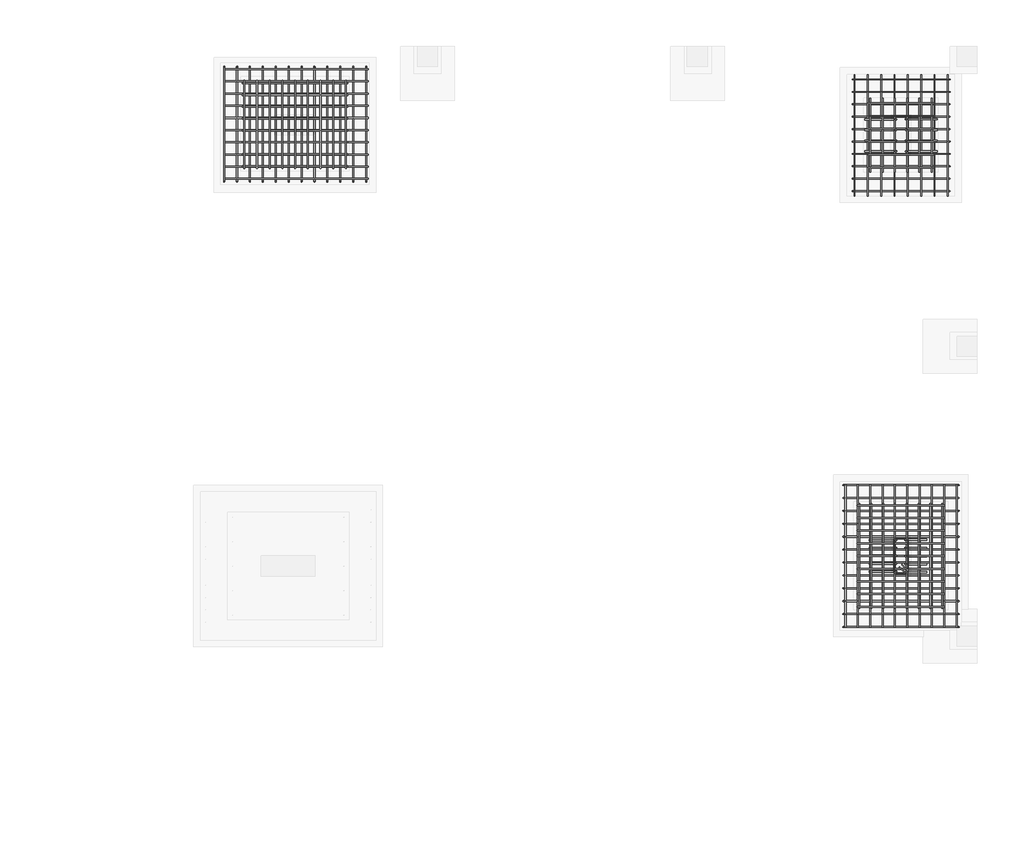
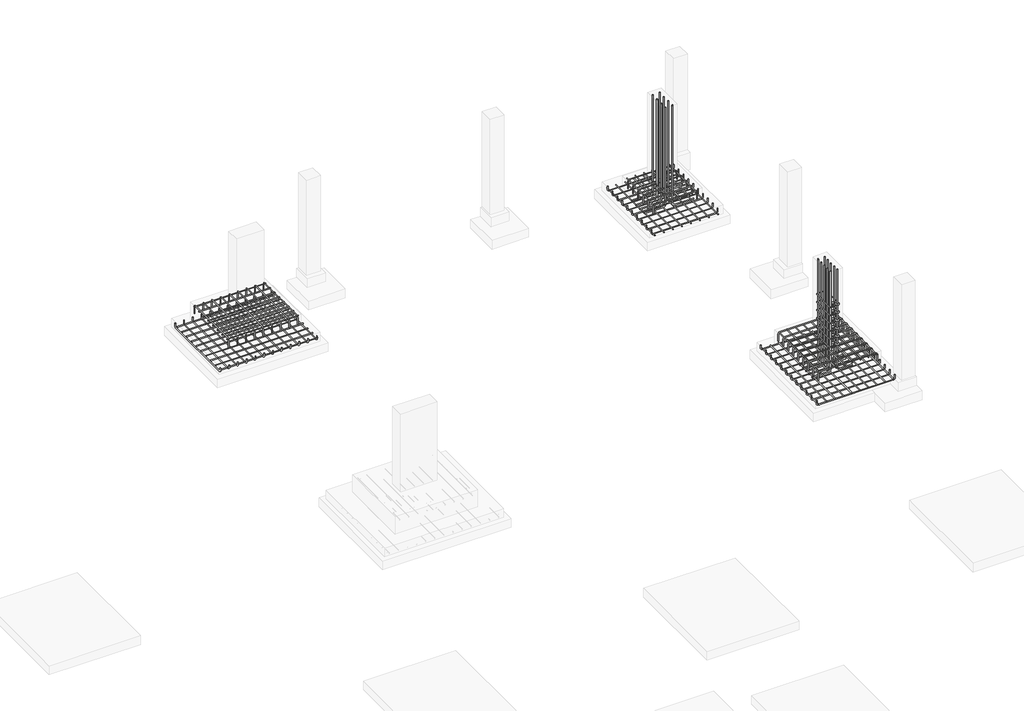
# One storey, part 6 of 6: 17 reinforcing bars.
"""IFC4 building model written with IfcOpenShell, lengths in millimetres."""

from ifc_helpers import new_model, si_unit, point, frame, origin, place, context, project, spatial, polyline, circle_curve, trimmed, segment, composite_curve, source, transform, mapped, element, save
from ifc_brep_helpers import swept_disk

model = new_model("IFC4")

# Units and contexts
model_context = context("Model", 3, world=origin())
ifc_project = project(units=[si_unit("LENGTHUNIT", "METRE", prefix="MILLI")], contexts=[model_context])

# Site, building, storey
site = spatial("IfcSite", under=ifc_project)
building = spatial("IfcBuilding", under=site)
storey = spatial("IfcBuildingStorey", under=building, Elevation=-1828.8)

# Reinforcing bars
placement = place(None, origin())
reinforcing_bar_shape = source(origin(), model_context, "Body", "SolidModel", [
    swept_disk(composite_curve([segment(polyline([(5668412.2527589, -3584746.7384702, -1801.3373708), (5670028.6527589, -3584746.7384702, -1801.3373708)]), True, "CONTINUOUS")], self_intersect=False), 6.0),
])
element("IfcReinforcingBar", 1, at=placement, inside=storey, context=model_context, shape_type="MappedRepresentation", body=[
    mapped(reinforcing_bar_shape, transform((0.0, 0.0, 0.0), x_axis=(1.0, 0.0, 0.0), y_axis=(0.0, 1.0, 0.0), z_axis=(0.0, 0.0, 1.0))),
    mapped(reinforcing_bar_shape, transform((0.0, -137.644158, 0.0), x_axis=(1.0, 0.0, 0.0), y_axis=(0.0, 1.0, 0.0), z_axis=(0.0, 0.0, 1.0))),
    mapped(reinforcing_bar_shape, transform((0.0, -275.2883159, 0.0), x_axis=(1.0, 0.0, 0.0), y_axis=(0.0, 1.0, 0.0), z_axis=(0.0, 0.0, 1.0))),
    mapped(reinforcing_bar_shape, transform((0.0, -412.9324739, 0.0), x_axis=(1.0, 0.0, 0.0), y_axis=(0.0, 1.0, 0.0), z_axis=(0.0, 0.0, 1.0))),
    mapped(reinforcing_bar_shape, transform((0.0, -550.5766318, 0.0), x_axis=(1.0, 0.0, 0.0), y_axis=(0.0, 1.0, 0.0), z_axis=(0.0, 0.0, 1.0))),
    mapped(reinforcing_bar_shape, transform((0.0, -688.2207898, 0.0), x_axis=(1.0, 0.0, 0.0), y_axis=(0.0, 1.0, 0.0), z_axis=(0.0, 0.0, 1.0))),
    mapped(reinforcing_bar_shape, transform((0.0, -825.8649477, 0.0), x_axis=(1.0, 0.0, 0.0), y_axis=(0.0, 1.0, 0.0), z_axis=(0.0, 0.0, 1.0))),
    mapped(reinforcing_bar_shape, transform((0.0, -963.5091057, 0.0), x_axis=(1.0, 0.0, 0.0), y_axis=(0.0, 1.0, 0.0), z_axis=(0.0, 0.0, 1.0))),
    mapped(reinforcing_bar_shape, transform((0.0, -1101.1532636, 0.0), x_axis=(1.0, 0.0, 0.0), y_axis=(0.0, 1.0, 0.0), z_axis=(0.0, 0.0, 1.0))),
    mapped(reinforcing_bar_shape, transform((0.0, -1238.7974216, 0.0), x_axis=(1.0, 0.0, 0.0), y_axis=(0.0, 1.0, 0.0), z_axis=(0.0, 0.0, 1.0))),
])
reinforcing_bar_2_shape = source(origin(), model_context, "Body", "SolidModel", [
    swept_disk(composite_curve([segment(polyline([(5669774.8297535, -3585864.1224803, -1551.6), (5669774.8297535, -3585864.1224803, -1437.6)]), True, "CONTINUOUS"), segment(trimmed(circle_curve(frame((5669774.8297535, -3585834.1224803, -1437.6), z_axis=(-1.0, 0.0, 0.0), x_axis=(0.0, -30.0, 0.0)), 30.0), [point((5669774.8297535, -3585864.1224803, -1437.6))], [point((5669774.8297535, -3585834.1224803, -1407.6))], True, "CARTESIAN"), True, "CONTINUOUS"), segment(polyline([(5669774.8297535, -3585834.1224803, -1407.6), (5669774.8297535, -3584907.6254563, -1407.6)]), True, "CONTINUOUS"), segment(trimmed(circle_curve(frame((5669774.8297535, -3584907.6254563, -1437.6), z_axis=(-1.0, 0.0, 0.0), x_axis=(0.0, 0.0, 30.0)), 30.0), [point((5669774.8297535, -3584907.6254563, -1407.6))], [point((5669774.8297535, -3584877.6254563, -1437.6))], True, "CARTESIAN"), True, "CONTINUOUS"), segment(polyline([(5669774.8297535, -3584877.6254563, -1437.6), (5669774.8297535, -3584877.6254563, -1551.6)]), True, "CONTINUOUS")], self_intersect=False), 6.0),
])
element("IfcReinforcingBar", 2, at=placement, inside=storey, context=model_context, shape_type="MappedRepresentation", body=[
    mapped(reinforcing_bar_2_shape, transform((0.0, 0.0, 0.0), x_axis=(1.0, 0.0, 0.0), y_axis=(0.0, 1.0, 0.0), z_axis=(0.0, 0.0, 1.0))),
    mapped(reinforcing_bar_2_shape, transform((-143.4, 0.0, 0.0), x_axis=(1.0, 0.0, 0.0), y_axis=(0.0, 1.0, 0.0), z_axis=(0.0, 0.0, 1.0))),
    mapped(reinforcing_bar_2_shape, transform((-286.8, 0.0, 0.0), x_axis=(1.0, 0.0, 0.0), y_axis=(0.0, 1.0, 0.0), z_axis=(0.0, 0.0, 1.0))),
    mapped(reinforcing_bar_2_shape, transform((-430.2, 0.0, 0.0), x_axis=(1.0, 0.0, 0.0), y_axis=(0.0, 1.0, 0.0), z_axis=(0.0, 0.0, 1.0))),
    mapped(reinforcing_bar_2_shape, transform((-573.6, 0.0, 0.0), x_axis=(1.0, 0.0, 0.0), y_axis=(0.0, 1.0, 0.0), z_axis=(0.0, 0.0, 1.0))),
    mapped(reinforcing_bar_2_shape, transform((-717.0, 0.0, 0.0), x_axis=(1.0, 0.0, 0.0), y_axis=(0.0, 1.0, 0.0), z_axis=(0.0, 0.0, 1.0))),
    mapped(reinforcing_bar_2_shape, transform((-860.4, 0.0, 0.0), x_axis=(1.0, 0.0, 0.0), y_axis=(0.0, 1.0, 0.0), z_axis=(0.0, 0.0, 1.0))),
    mapped(reinforcing_bar_2_shape, transform((-1003.8, 0.0, 0.0), x_axis=(1.0, 0.0, 0.0), y_axis=(0.0, 1.0, 0.0), z_axis=(0.0, 0.0, 1.0))),
    mapped(reinforcing_bar_2_shape, transform((-1147.2, 0.0, 0.0), x_axis=(1.0, 0.0, 0.0), y_axis=(0.0, 1.0, 0.0), z_axis=(0.0, 0.0, 1.0))),
])
reinforcing_bar_3_shape = source(origin(), model_context, "Body", "SolidModel", [
    swept_disk(composite_curve([segment(polyline([(5669794.2997613, -3585840.5657222, -1419.7151301), (5668606.7353359, -3585840.5657222, -1419.7151301)]), True, "CONTINUOUS")], self_intersect=False), 6.0),
])
element("IfcReinforcingBar", 3, at=placement, inside=storey, context=model_context, shape_type="MappedRepresentation", body=[
    mapped(reinforcing_bar_3_shape, transform((0.0, 0.0, 0.0), x_axis=(1.0, 0.0, 0.0), y_axis=(0.0, 1.0, 0.0), z_axis=(0.0, 0.0, 1.0))),
    mapped(reinforcing_bar_3_shape, transform((0.0, 133.8141, 0.0), x_axis=(1.0, 0.0, 0.0), y_axis=(0.0, 1.0, 0.0), z_axis=(0.0, 0.0, 1.0))),
    mapped(reinforcing_bar_3_shape, transform((0.0, 267.6282001, 0.0), x_axis=(1.0, 0.0, 0.0), y_axis=(0.0, 1.0, 0.0), z_axis=(0.0, 0.0, 1.0))),
    mapped(reinforcing_bar_3_shape, transform((0.0, 401.4423001, 0.0), x_axis=(1.0, 0.0, 0.0), y_axis=(0.0, 1.0, 0.0), z_axis=(0.0, 0.0, 1.0))),
    mapped(reinforcing_bar_3_shape, transform((0.0, 535.2564002, 0.0), x_axis=(1.0, 0.0, 0.0), y_axis=(0.0, 1.0, 0.0), z_axis=(0.0, 0.0, 1.0))),
    mapped(reinforcing_bar_3_shape, transform((0.0, 669.0705002, 0.0), x_axis=(1.0, 0.0, 0.0), y_axis=(0.0, 1.0, 0.0), z_axis=(0.0, 0.0, 1.0))),
    mapped(reinforcing_bar_3_shape, transform((0.0, 802.8846003, 0.0), x_axis=(1.0, 0.0, 0.0), y_axis=(0.0, 1.0, 0.0), z_axis=(0.0, 0.0, 1.0))),
    mapped(reinforcing_bar_3_shape, transform((0.0, 936.6987003, 0.0), x_axis=(1.0, 0.0, 0.0), y_axis=(0.0, 1.0, 0.0), z_axis=(0.0, 0.0, 1.0))),
])
reinforcing_bar_4_shape = source(origin(), model_context, "Body", "SolidModel", [
    swept_disk(composite_curve([segment(polyline([(5676673.9153747, -3589441.4682909, -1779.1123708), (5676673.9153747, -3591057.8682909, -1779.1123708)]), True, "CONTINUOUS")], self_intersect=False), 6.0),
])
element("IfcReinforcingBar", 4, at=placement, inside=storey, context=model_context, shape_type="MappedRepresentation", body=[
    mapped(reinforcing_bar_4_shape, transform((0.0, 0.0, 0.0), x_axis=(1.0, 0.0, 0.0), y_axis=(0.0, 1.0, 0.0), z_axis=(0.0, 0.0, 1.0))),
    mapped(reinforcing_bar_4_shape, transform((-139.3613026, 0.0, 0.0), x_axis=(1.0, 0.0, 0.0), y_axis=(0.0, 1.0, 0.0), z_axis=(0.0, 0.0, 1.0))),
    mapped(reinforcing_bar_4_shape, transform((-278.7226053, 0.0, 0.0), x_axis=(1.0, 0.0, 0.0), y_axis=(0.0, 1.0, 0.0), z_axis=(0.0, 0.0, 1.0))),
    mapped(reinforcing_bar_4_shape, transform((-418.0839079, 0.0, 0.0), x_axis=(1.0, 0.0, 0.0), y_axis=(0.0, 1.0, 0.0), z_axis=(0.0, 0.0, 1.0))),
    mapped(reinforcing_bar_4_shape, transform((-557.4452106, 0.0, 0.0), x_axis=(1.0, 0.0, 0.0), y_axis=(0.0, 1.0, 0.0), z_axis=(0.0, 0.0, 1.0))),
    mapped(reinforcing_bar_4_shape, transform((-696.8065132, 0.0, 0.0), x_axis=(1.0, 0.0, 0.0), y_axis=(0.0, 1.0, 0.0), z_axis=(0.0, 0.0, 1.0))),
    mapped(reinforcing_bar_4_shape, transform((-836.1678159, 0.0, 0.0), x_axis=(1.0, 0.0, 0.0), y_axis=(0.0, 1.0, 0.0), z_axis=(0.0, 0.0, 1.0))),
    mapped(reinforcing_bar_4_shape, transform((-975.5291185, 0.0, 0.0), x_axis=(1.0, 0.0, 0.0), y_axis=(0.0, 1.0, 0.0), z_axis=(0.0, 0.0, 1.0))),
    mapped(reinforcing_bar_4_shape, transform((-1114.8904212, 0.0, 0.0), x_axis=(1.0, 0.0, 0.0), y_axis=(0.0, 1.0, 0.0), z_axis=(0.0, 0.0, 1.0))),
    mapped(reinforcing_bar_4_shape, transform((-1254.2517238, 0.0, 0.0), x_axis=(1.0, 0.0, 0.0), y_axis=(0.0, 1.0, 0.0), z_axis=(0.0, 0.0, 1.0))),
])
reinforcing_bar_5_shape = source(origin(), model_context, "Body", "SolidModel", [
    swept_disk(composite_curve([segment(polyline([(5675555.1175203, -3590823.2682909, -1551.6), (5675555.1175203, -3590823.2682909, -1437.6)]), True, "CONTINUOUS"), segment(trimmed(circle_curve(frame((5675585.1175203, -3590823.2682909, -1437.6), z_axis=(0.0, 1.0, 0.0), x_axis=(-30.0, 0.0, 0.0)), 30.0), [point((5675555.1175203, -3590823.2682909, -1437.6))], [point((5675585.1175203, -3590823.2682909, -1407.6))], True, "CARTESIAN"), True, "CONTINUOUS"), segment(polyline([(5675585.1175203, -3590823.2682909, -1407.6), (5676504.297314, -3590823.2682909, -1407.6)]), True, "CONTINUOUS"), segment(trimmed(circle_curve(frame((5676504.297314, -3590823.2682909, -1437.6), z_axis=(0.0, 1.0, 0.0), x_axis=(0.0, 0.0, 30.0)), 30.0), [point((5676504.297314, -3590823.2682909, -1407.6))], [point((5676534.297314, -3590823.2682909, -1437.6))], True, "CARTESIAN"), True, "CONTINUOUS"), segment(polyline([(5676534.297314, -3590823.2682909, -1437.6), (5676534.297314, -3590823.2682909, -1551.6)]), True, "CONTINUOUS")], self_intersect=False), 6.0),
])
element("IfcReinforcingBar", 5, at=placement, inside=storey, context=model_context, shape_type="MappedRepresentation", body=[
    mapped(reinforcing_bar_5_shape, transform((0.0, 0.0, 0.0), x_axis=(1.0, 0.0, 0.0), y_axis=(0.0, 1.0, 0.0), z_axis=(0.0, 0.0, 1.0))),
    mapped(reinforcing_bar_5_shape, transform((0.0, 143.4, 0.0), x_axis=(1.0, 0.0, 0.0), y_axis=(0.0, 1.0, 0.0), z_axis=(0.0, 0.0, 1.0))),
    mapped(reinforcing_bar_5_shape, transform((0.0, 286.8, 0.0), x_axis=(1.0, 0.0, 0.0), y_axis=(0.0, 1.0, 0.0), z_axis=(0.0, 0.0, 1.0))),
    mapped(reinforcing_bar_5_shape, transform((0.0, 430.2, 0.0), x_axis=(1.0, 0.0, 0.0), y_axis=(0.0, 1.0, 0.0), z_axis=(0.0, 0.0, 1.0))),
    mapped(reinforcing_bar_5_shape, transform((0.0, 573.6, 0.0), x_axis=(1.0, 0.0, 0.0), y_axis=(0.0, 1.0, 0.0), z_axis=(0.0, 0.0, 1.0))),
    mapped(reinforcing_bar_5_shape, transform((0.0, 717.0, 0.0), x_axis=(1.0, 0.0, 0.0), y_axis=(0.0, 1.0, 0.0), z_axis=(0.0, 0.0, 1.0))),
    mapped(reinforcing_bar_5_shape, transform((0.0, 860.4, 0.0), x_axis=(1.0, 0.0, 0.0), y_axis=(0.0, 1.0, 0.0), z_axis=(0.0, 0.0, 1.0))),
    mapped(reinforcing_bar_5_shape, transform((0.0, 1003.8, 0.0), x_axis=(1.0, 0.0, 0.0), y_axis=(0.0, 1.0, 0.0), z_axis=(0.0, 0.0, 1.0))),
    mapped(reinforcing_bar_5_shape, transform((0.0, 1147.2, 0.0), x_axis=(1.0, 0.0, 0.0), y_axis=(0.0, 1.0, 0.0), z_axis=(0.0, 0.0, 1.0))),
])
reinforcing_bar_6_shape = source(origin(), model_context, "Body", "SolidModel", [
    swept_disk(composite_curve([segment(polyline([(5675575.9558156, -3590842.7382987, -1422.4932551), (5675575.9558156, -3589655.1738733, -1422.4932551)]), True, "CONTINUOUS")], self_intersect=False), 6.0),
])
element("IfcReinforcingBar", 6, at=placement, inside=storey, context=model_context, shape_type="MappedRepresentation", body=[
    mapped(reinforcing_bar_6_shape, transform((0.0, 0.0, 0.0), x_axis=(1.0, 0.0, 0.0), y_axis=(0.0, 1.0, 0.0), z_axis=(0.0, 0.0, 1.0))),
    mapped(reinforcing_bar_6_shape, transform((133.9163998, 0.0, 0.0), x_axis=(1.0, 0.0, 0.0), y_axis=(0.0, 1.0, 0.0), z_axis=(0.0, 0.0, 1.0))),
    mapped(reinforcing_bar_6_shape, transform((267.8327995, 0.0, 0.0), x_axis=(1.0, 0.0, 0.0), y_axis=(0.0, 1.0, 0.0), z_axis=(0.0, 0.0, 1.0))),
    mapped(reinforcing_bar_6_shape, transform((401.7491993, 0.0, 0.0), x_axis=(1.0, 0.0, 0.0), y_axis=(0.0, 1.0, 0.0), z_axis=(0.0, 0.0, 1.0))),
    mapped(reinforcing_bar_6_shape, transform((535.665599, 0.0, 0.0), x_axis=(1.0, 0.0, 0.0), y_axis=(0.0, 1.0, 0.0), z_axis=(0.0, 0.0, 1.0))),
    mapped(reinforcing_bar_6_shape, transform((669.5819988, 0.0, 0.0), x_axis=(1.0, 0.0, 0.0), y_axis=(0.0, 1.0, 0.0), z_axis=(0.0, 0.0, 1.0))),
    mapped(reinforcing_bar_6_shape, transform((803.4983986, 0.0, 0.0), x_axis=(1.0, 0.0, 0.0), y_axis=(0.0, 1.0, 0.0), z_axis=(0.0, 0.0, 1.0))),
    mapped(reinforcing_bar_6_shape, transform((937.4147983, 0.0, 0.0), x_axis=(1.0, 0.0, 0.0), y_axis=(0.0, 1.0, 0.0), z_axis=(0.0, 0.0, 1.0))),
])
reinforcing_bar_7_shape = source(origin(), model_context, "Body", "SolidModel", [
    swept_disk(composite_curve([segment(polyline([(5675396.7165246, -3589447.4682909, -1713.8), (5675396.7165246, -3589447.4682909, -1762.8)]), True, "CONTINUOUS"), segment(trimmed(circle_curve(frame((5675426.7165246, -3589447.4682909, -1762.8), z_axis=(0.0, -1.0, 0.0), x_axis=(-30.0, 0.0, 0.0)), 30.0), [point((5675396.7165246, -3589447.4682909, -1762.8))], [point((5675426.7165246, -3589447.4682909, -1792.8))], True, "CARTESIAN"), True, "CONTINUOUS"), segment(polyline([(5675426.7165246, -3589447.4682909, -1792.8), (5676666.3165246, -3589447.4682909, -1792.8)]), True, "CONTINUOUS"), segment(trimmed(circle_curve(frame((5676666.3165246, -3589447.4682909, -1762.8), z_axis=(0.0, -1.0, 0.0), x_axis=(0.0, 0.0, -30.0)), 30.0), [point((5676666.3165246, -3589447.4682909, -1792.8))], [point((5676696.3165246, -3589447.4682909, -1762.8))], True, "CARTESIAN"), True, "CONTINUOUS"), segment(polyline([(5676696.3165246, -3589447.4682909, -1762.8), (5676696.3165246, -3589447.4682909, -1713.8)]), True, "CONTINUOUS")], self_intersect=False), 6.0),
])
element("IfcReinforcingBar", 7, at=placement, inside=storey, context=model_context, shape_type="MappedRepresentation", body=[
    mapped(reinforcing_bar_7_shape, transform((0.0, 0.0, 0.0), x_axis=(1.0, 0.0, 0.0), y_axis=(0.0, 1.0, 0.0), z_axis=(0.0, 0.0, 1.0))),
    mapped(reinforcing_bar_7_shape, transform((0.0, -145.8545455, 0.0), x_axis=(1.0, 0.0, 0.0), y_axis=(0.0, 1.0, 0.0), z_axis=(0.0, 0.0, 1.0))),
    mapped(reinforcing_bar_7_shape, transform((0.0, -291.7090909, 0.0), x_axis=(1.0, 0.0, 0.0), y_axis=(0.0, 1.0, 0.0), z_axis=(0.0, 0.0, 1.0))),
    mapped(reinforcing_bar_7_shape, transform((0.0, -437.5636364, 0.0), x_axis=(1.0, 0.0, 0.0), y_axis=(0.0, 1.0, 0.0), z_axis=(0.0, 0.0, 1.0))),
    mapped(reinforcing_bar_7_shape, transform((0.0, -583.4181818, 0.0), x_axis=(1.0, 0.0, 0.0), y_axis=(0.0, 1.0, 0.0), z_axis=(0.0, 0.0, 1.0))),
    mapped(reinforcing_bar_7_shape, transform((0.0, -729.2727273, 0.0), x_axis=(1.0, 0.0, 0.0), y_axis=(0.0, 1.0, 0.0), z_axis=(0.0, 0.0, 1.0))),
    mapped(reinforcing_bar_7_shape, transform((0.0, -875.1272727, 0.0), x_axis=(1.0, 0.0, 0.0), y_axis=(0.0, 1.0, 0.0), z_axis=(0.0, 0.0, 1.0))),
    mapped(reinforcing_bar_7_shape, transform((0.0, -1020.9818182, 0.0), x_axis=(1.0, 0.0, 0.0), y_axis=(0.0, 1.0, 0.0), z_axis=(0.0, 0.0, 1.0))),
    mapped(reinforcing_bar_7_shape, transform((0.0, -1166.8363636, 0.0), x_axis=(1.0, 0.0, 0.0), y_axis=(0.0, 1.0, 0.0), z_axis=(0.0, 0.0, 1.0))),
    mapped(reinforcing_bar_7_shape, transform((0.0, -1312.6909091, 0.0), x_axis=(1.0, 0.0, 0.0), y_axis=(0.0, 1.0, 0.0), z_axis=(0.0, 0.0, 1.0))),
    mapped(reinforcing_bar_7_shape, transform((0.0, -1458.5454545, 0.0), x_axis=(1.0, 0.0, 0.0), y_axis=(0.0, 1.0, 0.0), z_axis=(0.0, 0.0, 1.0))),
    mapped(reinforcing_bar_7_shape, transform((0.0, -1604.4, 0.0), x_axis=(1.0, 0.0, 0.0), y_axis=(0.0, 1.0, 0.0), z_axis=(0.0, 0.0, 1.0))),
])
reinforcing_bar_8_shape = source(origin(), model_context, "Body", "SolidModel", [
    swept_disk(composite_curve([segment(polyline([(5675498.9545513, -3584862.9224803, -1738.4709043), (5675498.9545513, -3584862.9224803, -1793.4709043)]), True, "CONTINUOUS"), segment(trimmed(circle_curve(frame((5675523.9545513, -3584862.9224803, -1793.4709043), z_axis=(0.0, -1.0, 0.0), x_axis=(-25.0, 0.0, 0.0)), 25.0), [point((5675498.9545513, -3584862.9224803, -1793.4709043))], [point((5675523.9545513, -3584862.9224803, -1818.4709043))], True, "CARTESIAN"), True, "CONTINUOUS"), segment(polyline([(5675523.9545513, -3584862.9224803, -1818.4709043), (5676570.5431067, -3584862.9224803, -1818.4709043)]), True, "CONTINUOUS"), segment(trimmed(circle_curve(frame((5676570.5431067, -3584862.9224803, -1793.4709043), z_axis=(0.0, -1.0, 0.0), x_axis=(0.0, 0.0, -25.0)), 25.0), [point((5676570.5431067, -3584862.9224803, -1818.4709043))], [point((5676595.5431067, -3584862.9224803, -1793.4709043))], True, "CARTESIAN"), True, "CONTINUOUS"), segment(polyline([(5676595.5431067, -3584862.9224803, -1793.4709043), (5676595.5431067, -3584862.9224803, -1738.4709043)]), True, "CONTINUOUS")], self_intersect=False), 5.0),
])
element("IfcReinforcingBar", 8, at=placement, inside=storey, context=model_context, shape_type="MappedRepresentation", body=[
    mapped(reinforcing_bar_8_shape, transform((0.0, 0.0, 0.0), x_axis=(1.0, 0.0, 0.0), y_axis=(0.0, 1.0, 0.0), z_axis=(0.0, 0.0, 1.0))),
    mapped(reinforcing_bar_8_shape, transform((0.0, -140.1777778, 0.0), x_axis=(1.0, 0.0, 0.0), y_axis=(0.0, 1.0, 0.0), z_axis=(0.0, 0.0, 1.0))),
    mapped(reinforcing_bar_8_shape, transform((0.0, -280.3555556, 0.0), x_axis=(1.0, 0.0, 0.0), y_axis=(0.0, 1.0, 0.0), z_axis=(0.0, 0.0, 1.0))),
    mapped(reinforcing_bar_8_shape, transform((0.0, -420.5333333, 0.0), x_axis=(1.0, 0.0, 0.0), y_axis=(0.0, 1.0, 0.0), z_axis=(0.0, 0.0, 1.0))),
    mapped(reinforcing_bar_8_shape, transform((0.0, -560.7111111, 0.0), x_axis=(1.0, 0.0, 0.0), y_axis=(0.0, 1.0, 0.0), z_axis=(0.0, 0.0, 1.0))),
    mapped(reinforcing_bar_8_shape, transform((0.0, -700.8888889, 0.0), x_axis=(1.0, 0.0, 0.0), y_axis=(0.0, 1.0, 0.0), z_axis=(0.0, 0.0, 1.0))),
    mapped(reinforcing_bar_8_shape, transform((0.0, -841.0666667, 0.0), x_axis=(1.0, 0.0, 0.0), y_axis=(0.0, 1.0, 0.0), z_axis=(0.0, 0.0, 1.0))),
    mapped(reinforcing_bar_8_shape, transform((0.0, -981.2444444, 0.0), x_axis=(1.0, 0.0, 0.0), y_axis=(0.0, 1.0, 0.0), z_axis=(0.0, 0.0, 1.0))),
    mapped(reinforcing_bar_8_shape, transform((0.0, -1121.4222222, 0.0), x_axis=(1.0, 0.0, 0.0), y_axis=(0.0, 1.0, 0.0), z_axis=(0.0, 0.0, 1.0))),
    mapped(reinforcing_bar_8_shape, transform((0.0, -1261.6, 0.0), x_axis=(1.0, 0.0, 0.0), y_axis=(0.0, 1.0, 0.0), z_axis=(0.0, 0.0, 1.0))),
])
reinforcing_bar_9_shape = source(origin(), model_context, "Body", "SolidModel", [
    swept_disk(composite_curve([segment(polyline([(5676410.6165246, -3585129.6224803, -1673.2), (5676410.6165246, -3585129.6224803, -1553.2)]), True, "CONTINUOUS"), segment(trimmed(circle_curve(frame((5676385.6165246, -3585129.6224803, -1553.2), z_axis=(0.0, -1.0, 0.0), x_axis=(25.0, 0.0, 0.0)), 25.0), [point((5676410.6165246, -3585129.6224803, -1553.2))], [point((5676385.6165246, -3585129.6224803, -1528.2))], True, "CARTESIAN"), True, "CONTINUOUS"), segment(polyline([(5676385.6165246, -3585129.6224803, -1528.2), (5675707.4165246, -3585129.6224803, -1528.2)]), True, "CONTINUOUS"), segment(trimmed(circle_curve(frame((5675707.4165246, -3585129.6224803, -1553.2), z_axis=(0.0, -1.0, 0.0), x_axis=(0.0, 0.0, 25.0)), 25.0), [point((5675707.4165246, -3585129.6224803, -1528.2))], [point((5675682.4165246, -3585129.6224803, -1553.2))], True, "CARTESIAN"), True, "CONTINUOUS"), segment(polyline([(5675682.4165246, -3585129.6224803, -1553.2), (5675682.4165246, -3585129.6224803, -1673.2)]), True, "CONTINUOUS")], self_intersect=False), 5.0),
])
element("IfcReinforcingBar", 9, at=placement, inside=storey, context=model_context, shape_type="MappedRepresentation", body=[
    mapped(reinforcing_bar_9_shape, transform((0.0, 0.0, 0.0), x_axis=(1.0, 0.0, 0.0), y_axis=(0.0, 1.0, 0.0), z_axis=(0.0, 0.0, 1.0))),
    mapped(reinforcing_bar_9_shape, transform((0.0, -145.64, 0.0), x_axis=(1.0, 0.0, 0.0), y_axis=(0.0, 1.0, 0.0), z_axis=(0.0, 0.0, 1.0))),
    mapped(reinforcing_bar_9_shape, transform((0.0, -291.28, 0.0), x_axis=(1.0, 0.0, 0.0), y_axis=(0.0, 1.0, 0.0), z_axis=(0.0, 0.0, 1.0))),
    mapped(reinforcing_bar_9_shape, transform((0.0, -436.92, 0.0), x_axis=(1.0, 0.0, 0.0), y_axis=(0.0, 1.0, 0.0), z_axis=(0.0, 0.0, 1.0))),
    mapped(reinforcing_bar_9_shape, transform((0.0, -582.56, 0.0), x_axis=(1.0, 0.0, 0.0), y_axis=(0.0, 1.0, 0.0), z_axis=(0.0, 0.0, 1.0))),
    mapped(reinforcing_bar_9_shape, transform((0.0, -728.2, 0.0), x_axis=(1.0, 0.0, 0.0), y_axis=(0.0, 1.0, 0.0), z_axis=(0.0, 0.0, 1.0))),
])
reinforcing_bar_10_shape = source(origin(), model_context, "Body", "SolidModel", [
    swept_disk(composite_curve([segment(polyline([(5675520.5984903, -3584807.9224803, -1807.7638193), (5675520.5984903, -3586179.5224803, -1807.7638193)]), True, "CONTINUOUS")], self_intersect=False), 5.0),
])
element("IfcReinforcingBar", 10, at=placement, inside=storey, context=model_context, shape_type="MappedRepresentation", body=[
    mapped(reinforcing_bar_10_shape, transform((0.0, 0.0, 0.0), x_axis=(1.0, 0.0, 0.0), y_axis=(0.0, 1.0, 0.0), z_axis=(0.0, 0.0, 1.0))),
    mapped(reinforcing_bar_10_shape, transform((150.6667583, 0.0, 0.0), x_axis=(1.0, 0.0, 0.0), y_axis=(0.0, 1.0, 0.0), z_axis=(0.0, 0.0, 1.0))),
    mapped(reinforcing_bar_10_shape, transform((301.3335165, 0.0, 0.0), x_axis=(1.0, 0.0, 0.0), y_axis=(0.0, 1.0, 0.0), z_axis=(0.0, 0.0, 1.0))),
    mapped(reinforcing_bar_10_shape, transform((452.0002748, 0.0, 0.0), x_axis=(1.0, 0.0, 0.0), y_axis=(0.0, 1.0, 0.0), z_axis=(0.0, 0.0, 1.0))),
    mapped(reinforcing_bar_10_shape, transform((602.6670331, 0.0, 0.0), x_axis=(1.0, 0.0, 0.0), y_axis=(0.0, 1.0, 0.0), z_axis=(0.0, 0.0, 1.0))),
    mapped(reinforcing_bar_10_shape, transform((753.3337913, 0.0, 0.0), x_axis=(1.0, 0.0, 0.0), y_axis=(0.0, 1.0, 0.0), z_axis=(0.0, 0.0, 1.0))),
    mapped(reinforcing_bar_10_shape, transform((904.0005496, 0.0, 0.0), x_axis=(1.0, 0.0, 0.0), y_axis=(0.0, 1.0, 0.0), z_axis=(0.0, 0.0, 1.0))),
    mapped(reinforcing_bar_10_shape, transform((1054.6673079, 0.0, 0.0), x_axis=(1.0, 0.0, 0.0), y_axis=(0.0, 1.0, 0.0), z_axis=(0.0, 0.0, 1.0))),
])
reinforcing_bar_11_shape = source(origin(), model_context, "Body", "SolidModel", [
    swept_disk(composite_curve([segment(polyline([(5676393.2066857, -3585074.6224803, -1540.036299), (5676393.2066857, -3585912.8224803, -1540.036299)]), True, "CONTINUOUS")], self_intersect=False), 5.0),
])
element("IfcReinforcingBar", 11, at=placement, inside=storey, context=model_context, shape_type="MappedRepresentation", body=[
    mapped(reinforcing_bar_11_shape, transform((0.0, 0.0, 0.0), x_axis=(1.0, 0.0, 0.0), y_axis=(0.0, 1.0, 0.0), z_axis=(0.0, 0.0, 1.0))),
    mapped(reinforcing_bar_11_shape, transform((-138.6844386, 0.0, 0.0), x_axis=(1.0, 0.0, 0.0), y_axis=(0.0, 1.0, 0.0), z_axis=(0.0, 0.0, 1.0))),
    mapped(reinforcing_bar_11_shape, transform((-277.3688772, 0.0, 0.0), x_axis=(1.0, 0.0, 0.0), y_axis=(0.0, 1.0, 0.0), z_axis=(0.0, 0.0, 1.0))),
    mapped(reinforcing_bar_11_shape, transform((-416.0533158, 0.0, 0.0), x_axis=(1.0, 0.0, 0.0), y_axis=(0.0, 1.0, 0.0), z_axis=(0.0, 0.0, 1.0))),
    mapped(reinforcing_bar_11_shape, transform((-554.7377544, 0.0, 0.0), x_axis=(1.0, 0.0, 0.0), y_axis=(0.0, 1.0, 0.0), z_axis=(0.0, 0.0, 1.0))),
    mapped(reinforcing_bar_11_shape, transform((-693.422193, 0.0, 0.0), x_axis=(1.0, 0.0, 0.0), y_axis=(0.0, 1.0, 0.0), z_axis=(0.0, 0.0, 1.0))),
])
reinforcing_bar_12_shape = source(origin(), model_context, "Body", "SolidModel", [
    swept_disk(composite_curve([segment(polyline([(5670003.4297535, -3584716.9224803, -1743.8), (5670003.4297535, -3584716.9224803, -1784.1059723)]), True, "CONTINUOUS"), segment(trimmed(circle_curve(frame((5670003.4297535, -3584746.9224803, -1784.1059723), z_axis=(-1.0, 0.0, 0.0), x_axis=(0.0, 30.0, 0.0)), 30.0), [point((5670003.4297535, -3584716.9224803, -1784.1059723))], [point((5670003.4297535, -3584746.9224803, -1814.1059723))], True, "CARTESIAN"), True, "CONTINUOUS"), segment(polyline([(5670003.4297535, -3584746.9224803, -1814.1059723), (5670003.4297535, -3585986.5224803, -1814.1059723)]), True, "CONTINUOUS"), segment(trimmed(circle_curve(frame((5670003.4297535, -3585986.5224803, -1784.1059723), z_axis=(-1.0, 0.0, 0.0), x_axis=(0.0, 0.0, -30.0)), 30.0), [point((5670003.4297535, -3585986.5224803, -1814.1059723))], [point((5670003.4297535, -3586016.5224803, -1784.1059723))], True, "CARTESIAN"), True, "CONTINUOUS"), segment(polyline([(5670003.4297535, -3586016.5224803, -1784.1059723), (5670003.4297535, -3586016.5224803, -1743.8)]), True, "CONTINUOUS")], self_intersect=False), 6.0),
])
element("IfcReinforcingBar", 12, at=placement, inside=storey, context=model_context, shape_type="MappedRepresentation", body=[
    mapped(reinforcing_bar_12_shape, transform((0.0, 0.0, 0.0), x_axis=(1.0, 0.0, 0.0), y_axis=(0.0, 1.0, 0.0), z_axis=(0.0, 0.0, 1.0))),
    mapped(reinforcing_bar_12_shape, transform((-145.8545455, 0.0, 0.0), x_axis=(1.0, 0.0, 0.0), y_axis=(0.0, 1.0, 0.0), z_axis=(0.0, 0.0, 1.0))),
    mapped(reinforcing_bar_12_shape, transform((-291.7090909, 0.0, 0.0), x_axis=(1.0, 0.0, 0.0), y_axis=(0.0, 1.0, 0.0), z_axis=(0.0, 0.0, 1.0))),
    mapped(reinforcing_bar_12_shape, transform((-437.5636364, 0.0, 0.0), x_axis=(1.0, 0.0, 0.0), y_axis=(0.0, 1.0, 0.0), z_axis=(0.0, 0.0, 1.0))),
    mapped(reinforcing_bar_12_shape, transform((-583.4181818, 0.0, 0.0), x_axis=(1.0, 0.0, 0.0), y_axis=(0.0, 1.0, 0.0), z_axis=(0.0, 0.0, 1.0))),
    mapped(reinforcing_bar_12_shape, transform((-729.2727273, 0.0, 0.0), x_axis=(1.0, 0.0, 0.0), y_axis=(0.0, 1.0, 0.0), z_axis=(0.0, 0.0, 1.0))),
    mapped(reinforcing_bar_12_shape, transform((-875.1272727, 0.0, 0.0), x_axis=(1.0, 0.0, 0.0), y_axis=(0.0, 1.0, 0.0), z_axis=(0.0, 0.0, 1.0))),
    mapped(reinforcing_bar_12_shape, transform((-1020.9818182, 0.0, 0.0), x_axis=(1.0, 0.0, 0.0), y_axis=(0.0, 1.0, 0.0), z_axis=(0.0, 0.0, 1.0))),
    mapped(reinforcing_bar_12_shape, transform((-1166.8363636, 0.0, 0.0), x_axis=(1.0, 0.0, 0.0), y_axis=(0.0, 1.0, 0.0), z_axis=(0.0, 0.0, 1.0))),
    mapped(reinforcing_bar_12_shape, transform((-1312.6909091, 0.0, 0.0), x_axis=(1.0, 0.0, 0.0), y_axis=(0.0, 1.0, 0.0), z_axis=(0.0, 0.0, 1.0))),
    mapped(reinforcing_bar_12_shape, transform((-1458.5454545, 0.0, 0.0), x_axis=(1.0, 0.0, 0.0), y_axis=(0.0, 1.0, 0.0), z_axis=(0.0, 0.0, 1.0))),
    mapped(reinforcing_bar_12_shape, transform((-1604.4, 0.0, 0.0), x_axis=(1.0, 0.0, 0.0), y_axis=(0.0, 1.0, 0.0), z_axis=(0.0, 0.0, 1.0))),
])
reinforcing_bar_13_shape = source(origin(), model_context, "Body", "SolidModel", [
    swept_disk(composite_curve([segment(polyline([(5676103.6665246, -3585311.1224803, -30.0), (5676103.6665246, -3585311.1224803, -1753.5240858)]), True, "CONTINUOUS"), segment(trimmed(circle_curve(frame((5676143.6665246, -3585311.1224803, -1753.5240858), z_axis=(0.0, -1.0, 0.0), x_axis=(-40.0, 0.0, 0.0)), 40.0), [point((5676103.6665246, -3585311.1224803, -1753.5240858))], [point((5676143.6665246, -3585311.1224803, -1793.5240858))], True, "CARTESIAN"), True, "CONTINUOUS"), segment(polyline([(5676143.6665246, -3585311.1224803, -1793.5240858), (5676458.3151188, -3585311.1224803, -1793.5240858)]), True, "CONTINUOUS")], self_intersect=False), 8.0),
])
element("IfcReinforcingBar", 13, at=placement, inside=storey, context=model_context, shape_type="MappedRepresentation", body=[
    mapped(reinforcing_bar_13_shape, transform((0.0, 0.0, 0.0), x_axis=(1.0, 0.0, 0.0), y_axis=(0.0, 1.0, 0.0), z_axis=(0.0, 0.0, 1.0))),
    mapped(reinforcing_bar_13_shape, transform((0.0, -121.7333333, 0.0), x_axis=(1.0, 0.0, 0.0), y_axis=(0.0, 1.0, 0.0), z_axis=(0.0, 0.0, 1.0))),
    mapped(reinforcing_bar_13_shape, transform((0.0, -243.4666667, 0.0), x_axis=(1.0, 0.0, 0.0), y_axis=(0.0, 1.0, 0.0), z_axis=(0.0, 0.0, 1.0))),
    mapped(reinforcing_bar_13_shape, transform((0.0, -365.2, 0.0), x_axis=(1.0, 0.0, 0.0), y_axis=(0.0, 1.0, 0.0), z_axis=(0.0, 0.0, 1.0))),
])
reinforcing_bar_14_shape = source(origin(), model_context, "Body", "SolidModel", [
    swept_disk(composite_curve([segment(polyline([(5675989.3665246, -3585313.9085925, -30.0), (5675989.3665246, -3585313.9085925, -1726.4720204)]), True, "CONTINUOUS"), segment(trimmed(circle_curve(frame((5675949.3665246, -3585313.9085925, -1726.4720204), z_axis=(0.0, 1.0, 0.0), x_axis=(40.0, 0.0, 0.0)), 40.0), [point((5675989.3665246, -3585313.9085925, -1726.4720204))], [point((5675949.3665246, -3585313.9085925, -1766.4720204))], True, "CARTESIAN"), True, "CONTINUOUS"), segment(polyline([(5675949.3665246, -3585313.9085925, -1766.4720204), (5675637.9027685, -3585313.9085925, -1766.4720204)]), True, "CONTINUOUS")], self_intersect=False), 8.0),
])
element("IfcReinforcingBar", 14, at=placement, inside=storey, context=model_context, shape_type="MappedRepresentation", body=[
    mapped(reinforcing_bar_14_shape, transform((0.0, 0.0, 0.0), x_axis=(1.0, 0.0, 0.0), y_axis=(0.0, 1.0, 0.0), z_axis=(0.0, 0.0, 1.0))),
    mapped(reinforcing_bar_14_shape, transform((0.0, -120.1712362, 0.0), x_axis=(1.0, 0.0, 0.0), y_axis=(0.0, 1.0, 0.0), z_axis=(0.0, 0.0, 1.0))),
    mapped(reinforcing_bar_14_shape, transform((0.0, -240.3424723, 0.0), x_axis=(1.0, 0.0, 0.0), y_axis=(0.0, 1.0, 0.0), z_axis=(0.0, 0.0, 1.0))),
    mapped(reinforcing_bar_14_shape, transform((0.0, -360.5137085, 0.0), x_axis=(1.0, 0.0, 0.0), y_axis=(0.0, 1.0, 0.0), z_axis=(0.0, 0.0, 1.0))),
])
reinforcing_bar_15_shape = source(origin(), model_context, "Body", "SolidModel", [
    swept_disk(composite_curve([segment(polyline([(5676097.3165246, -3590067.0682909, -30.0), (5676097.3165246, -3590067.0682909, -1746.25)]), True, "CONTINUOUS"), segment(trimmed(circle_curve(frame((5676137.3165246, -3590067.0682909, -1746.25), z_axis=(0.0, -1.0, 0.0), x_axis=(-40.0, 0.0, 0.0)), 40.0), [point((5676097.3165246, -3590067.0682909, -1746.25))], [point((5676137.3165246, -3590067.0682909, -1786.25))], True, "CARTESIAN"), True, "CONTINUOUS"), segment(polyline([(5676137.3165246, -3590067.0682909, -1786.25), (5676338.6702744, -3590067.0682909, -1786.25)]), True, "CONTINUOUS")], self_intersect=False), 8.0),
])
element("IfcReinforcingBar", 15, at=placement, inside=storey, context=model_context, shape_type="MappedRepresentation", body=[
    mapped(reinforcing_bar_15_shape, transform((0.0, 0.0, 0.0), x_axis=(1.0, 0.0, 0.0), y_axis=(0.0, 1.0, 0.0), z_axis=(0.0, 0.0, 1.0))),
    mapped(reinforcing_bar_15_shape, transform((0.0, -91.3, 0.0), x_axis=(1.0, 0.0, 0.0), y_axis=(0.0, 1.0, 0.0), z_axis=(0.0, 0.0, 1.0))),
    mapped(reinforcing_bar_15_shape, transform((0.0, -182.6, 0.0), x_axis=(1.0, 0.0, 0.0), y_axis=(0.0, 1.0, 0.0), z_axis=(0.0, 0.0, 1.0))),
    mapped(reinforcing_bar_15_shape, transform((0.0, -273.9, 0.0), x_axis=(1.0, 0.0, 0.0), y_axis=(0.0, 1.0, 0.0), z_axis=(0.0, 0.0, 1.0))),
    mapped(reinforcing_bar_15_shape, transform((0.0, -365.2, 0.0), x_axis=(1.0, 0.0, 0.0), y_axis=(0.0, 1.0, 0.0), z_axis=(0.0, 0.0, 1.0))),
])
reinforcing_bar_16_shape = source(origin(), model_context, "Body", "SolidModel", [
    swept_disk(composite_curve([segment(polyline([(5675988.8930234, -3590069.7988123, -30.0), (5675988.8930234, -3590069.7988123, -1745.1487332)]), True, "CONTINUOUS"), segment(trimmed(circle_curve(frame((5675948.8930234, -3590069.7988123, -1745.1487332), z_axis=(0.0, 1.0, 0.0), x_axis=(40.0, 0.0, 0.0)), 40.0), [point((5675988.8930234, -3590069.7988123, -1745.1487332))], [point((5675948.8930234, -3590069.7988123, -1785.1487332))], True, "CARTESIAN"), True, "CONTINUOUS"), segment(polyline([(5675948.8930234, -3590069.7988123, -1785.1487332), (5675685.3738958, -3590069.7988123, -1785.1487332)]), True, "CONTINUOUS")], self_intersect=False), 8.0),
])
element("IfcReinforcingBar", 16, at=placement, inside=storey, context=model_context, shape_type="MappedRepresentation", body=[
    mapped(reinforcing_bar_16_shape, transform((0.0, 0.0, 0.0), x_axis=(1.0, 0.0, 0.0), y_axis=(0.0, 1.0, 0.0), z_axis=(0.0, 0.0, 1.0))),
    mapped(reinforcing_bar_16_shape, transform((0.0, -88.7142136, 0.0), x_axis=(1.0, 0.0, 0.0), y_axis=(0.0, 1.0, 0.0), z_axis=(0.0, 0.0, 1.0))),
    mapped(reinforcing_bar_16_shape, transform((0.0, -177.4284271, 0.0), x_axis=(1.0, 0.0, 0.0), y_axis=(0.0, 1.0, 0.0), z_axis=(0.0, 0.0, 1.0))),
    mapped(reinforcing_bar_16_shape, transform((0.0, -266.1426407, 0.0), x_axis=(1.0, 0.0, 0.0), y_axis=(0.0, 1.0, 0.0), z_axis=(0.0, 0.0, 1.0))),
    mapped(reinforcing_bar_16_shape, transform((0.0, -354.8568543, 0.0), x_axis=(1.0, 0.0, 0.0), y_axis=(0.0, 1.0, 0.0), z_axis=(0.0, 0.0, 1.0))),
])
reinforcing_bar_17_shape = source(origin(), model_context, "Body", "SolidModel", [
    swept_disk(composite_curve([segment(polyline([(5676028.3276719, -3590374.0637095, -1337.6), (5676092.6743889, -3590438.4104266, -1337.6)]), True, "CONTINUOUS"), segment(trimmed(circle_curve(frame((5676106.8165246, -3590424.2682909, -1337.6), z_axis=(0.0, 0.0, 1.0), x_axis=(-14.142135699279606, -14.142135699745268, 0.0)), 20.0), [point((5676092.6743889, -3590438.4104266, -1337.6))], [point((5676126.8165246, -3590424.2682909, -1337.6))], True, "CARTESIAN"), True, "CONTINUOUS"), segment(polyline([(5676126.8165246, -3590424.2682909, -1337.6), (5676126.8165246, -3590075.0682909, -1337.6)]), True, "CONTINUOUS"), segment(trimmed(circle_curve(frame((5676106.8165246, -3590075.0682909, -1337.6), z_axis=(0.0, 0.0, 1.0), x_axis=(20.0, 0.0, 0.0)), 20.0), [point((5676126.8165246, -3590075.0682909, -1337.6))], [point((5676106.8165246, -3590055.0682909, -1337.6))], True, "CARTESIAN"), True, "CONTINUOUS"), segment(polyline([(5676106.8165246, -3590055.0682909, -1337.6), (5675986.2165246, -3590055.0682909, -1337.6)]), True, "CONTINUOUS"), segment(trimmed(circle_curve(frame((5675986.2165246, -3590075.0640672, -1338.0110129), z_axis=(0.0, -0.020550643642767298, 0.9997888132230066), x_axis=(0.0, 19.995776299852878, 0.41101290000005974)), 20.0), [point((5675986.2165246, -3590055.0682909, -1337.6))], [point((5675966.2165246, -3590075.0640672, -1338.0110129))], True, "CARTESIAN"), True, "CONTINUOUS"), segment(polyline([(5675966.2165246, -3590075.0640672, -1338.0110129), (5675966.2165246, -3590424.2725147, -1345.1889871)]), True, "CONTINUOUS"), segment(trimmed(circle_curve(frame((5675986.2165246, -3590424.2725147, -1345.1889871), z_axis=(0.0, -0.020550643642767298, 0.9997888132230066), x_axis=(-20.0, 0.0, 0.0)), 20.0), [point((5675966.2165246, -3590424.2725147, -1345.1889871))], [point((5675986.2165246, -3590444.2682909, -1345.6))], True, "CARTESIAN"), True, "CONTINUOUS"), segment(polyline([(5675986.2165246, -3590444.2682909, -1345.6), (5676106.8165246, -3590444.2682909, -1345.6)]), True, "CONTINUOUS"), segment(trimmed(circle_curve(frame((5676106.8165246, -3590424.2682909, -1345.6), z_axis=(0.0, 0.0, 1.0), x_axis=(0.0, -20.0, 0.0)), 20.0), [point((5676106.8165246, -3590444.2682909, -1345.6))], [point((5676120.9586602, -3590410.1261553, -1345.6))], True, "CARTESIAN"), True, "CONTINUOUS"), segment(polyline([(5676120.9586602, -3590410.1261553, -1345.6), (5676056.6119431, -3590345.7794382, -1345.6)]), True, "CONTINUOUS")], self_intersect=False), 4.0),
])
element("IfcReinforcingBar", 17, at=placement, inside=storey, context=model_context, shape_type="MappedRepresentation", body=[
    mapped(reinforcing_bar_17_shape, transform((0.0, 0.0, 0.0), x_axis=(1.0, 0.0, 0.0), y_axis=(0.0, 1.0, 0.0), z_axis=(0.0, 0.0, 1.0))),
    mapped(reinforcing_bar_17_shape, transform((0.0, 0.0, 140.101104), x_axis=(1.0, 0.0, 0.0), y_axis=(0.0, 1.0, 0.0), z_axis=(0.0, 0.0, 1.0))),
    mapped(reinforcing_bar_17_shape, transform((0.0, 0.0, 280.2022081), x_axis=(1.0, 0.0, 0.0), y_axis=(0.0, 1.0, 0.0), z_axis=(0.0, 0.0, 1.0))),
    mapped(reinforcing_bar_17_shape, transform((0.0, 0.0, 420.3033121), x_axis=(1.0, 0.0, 0.0), y_axis=(0.0, 1.0, 0.0), z_axis=(0.0, 0.0, 1.0))),
    mapped(reinforcing_bar_17_shape, transform((0.0, 0.0, 560.4044161), x_axis=(1.0, 0.0, 0.0), y_axis=(0.0, 1.0, 0.0), z_axis=(0.0, 0.0, 1.0))),
    mapped(reinforcing_bar_17_shape, transform((0.0, 0.0, 700.5055202), x_axis=(1.0, 0.0, 0.0), y_axis=(0.0, 1.0, 0.0), z_axis=(0.0, 0.0, 1.0))),
])

save(model, "model.ifc")

# Revit data of these elements
# Elements 1, 2, 3, 4, 5, 6, 7, 8, 9, 10, 11, 12, 13, 14, 15, 16, 17 (IfcReinforcingBar)
#   Phase Created = New Construction
